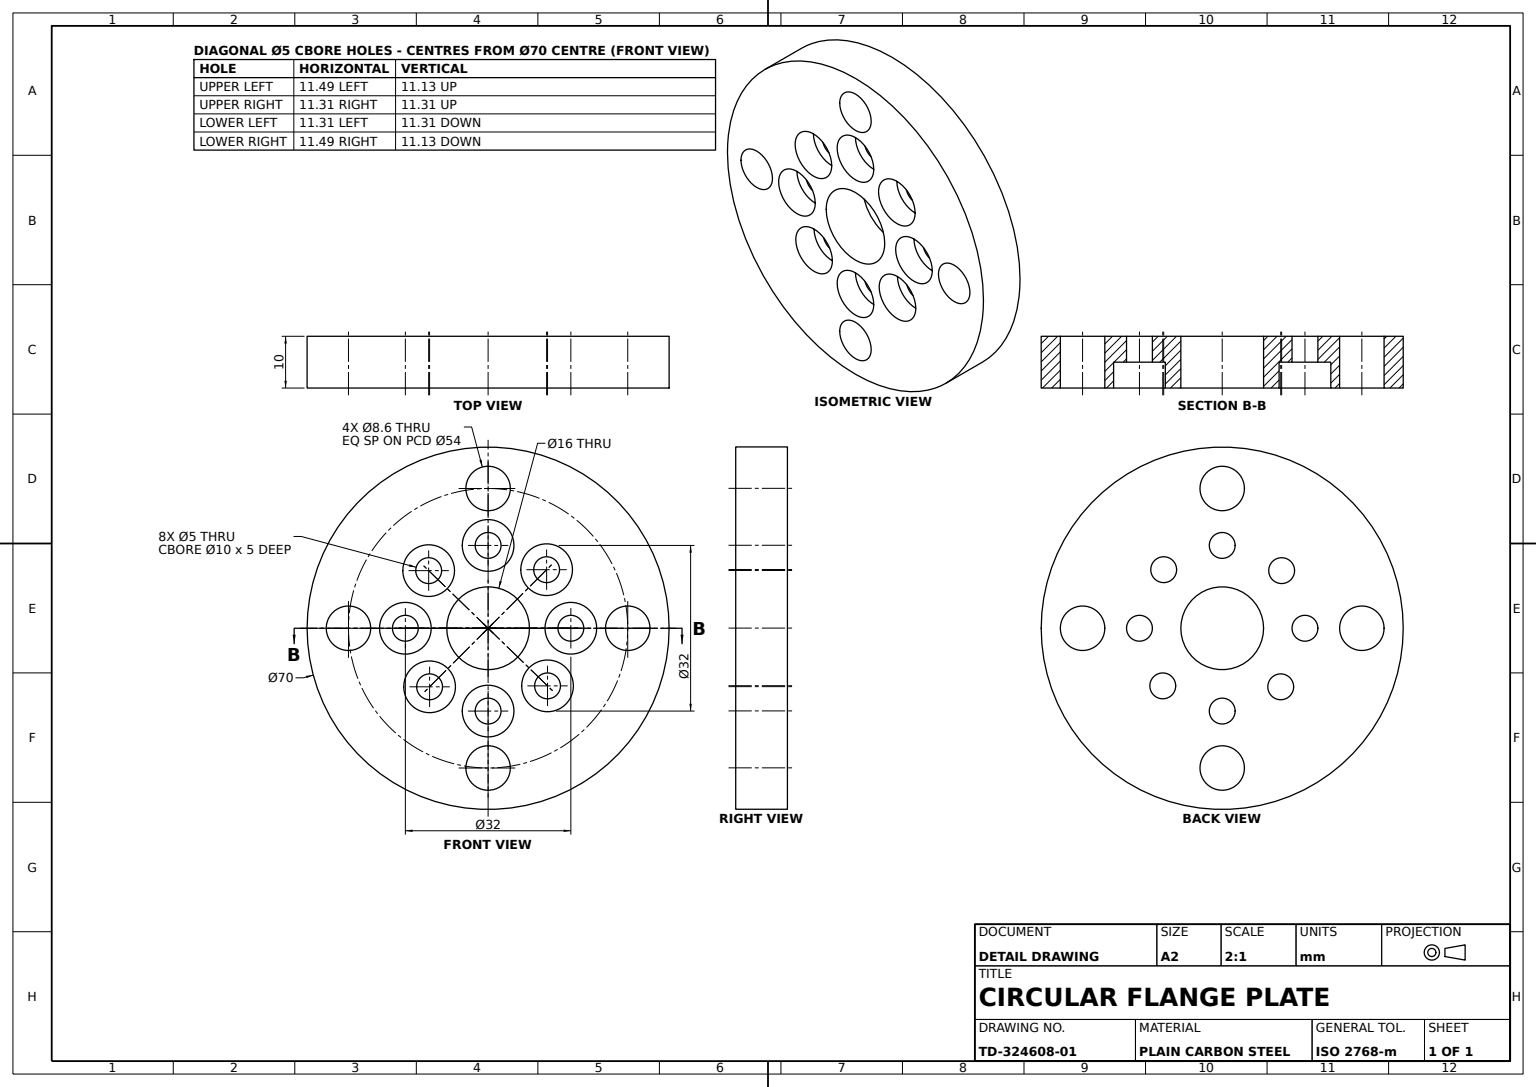
SolidWorks part; units mm, degrees
material "Plain Carbon Steel"
ref_plane "Front Plane" through (0, 0, 0) normal (0, 0, 1) x (1, 0, 0)
ref_plane "Top Plane" through (0, 0, 0) normal (0, 1, 0) x (1, 0, 0)
ref_plane "Right Plane" through (0, 0, 0) normal (1, 0, 0) x (0, 0, -1)
sketch "Disc Profile Ø70" plane through (0, 0, 0) normal (0, 0, 1) x (1, 0, 0)
  circle A0 centre (0, 0) radius 35
  dimension "D1" = 70
  dimension "D2" = 70
extrude "Disc Ø70 x 10" add sketch "Disc Profile Ø70" along normal blind 10
sketch "Centre Bore Profile Ø16" plane through (0, 0, 10) normal (0, 0, 1) x (1, 0, 0)
  circle A0 centre (0, 0) radius 8
  dimension "D1" = 16
  dimension "D2" = 16
extrude "Centre Bore Ø16" cut sketch "Centre Bore Profile Ø16" against normal blind 10
sketch "Outer Holes Profile 4xØ8.6" plane through (0, 0, 10) normal (0, 0, 1) x (1, 0, 0)
  circle A1 centre (0, 27) radius 4.3
  circle A2 centre (27, 0) radius 4.3
  circle A3 centre (0, -27) radius 4.3
  circle A4 centre (-27, 0) radius 4.3
  dimension "D1" = 8.6
  dimension "D2" = 8.6
  dimension "D3" = 8.6
  dimension "D4" = 8.6
  dimension "D5" = 8.6
  dimension "D6" = 27
  dimension "D7" = 27
  dimension "D8" = 27
  dimension "D9" = 27
extrude "Outer Holes 4xØ8.6" cut sketch "Outer Holes Profile 4xØ8.6" against normal blind 10
sketch "Counterbore Profile" plane through (0, 0, 10) normal (0, 0, 1) x (1, 0, 0)
  line L1 (0, 0) -> (0.0257, 0) construction
  line L3 (0, 0) -> (0.0086, 0) construction
  circle A1 centre (0, 16) radius 5
  circle A2 centre (16, 0) radius 5
  circle A3 centre (0, -16) radius 5
  circle A4 centre (-16, 0) radius 5
  circle A5 centre (11.4925, -11.132) radius 5
  circle A6 centre (11.3137, 11.3137) radius 5
  circle A7 centre (-11.4925, 11.132) radius 5
  circle A8 centre (-11.3137, -11.3137) radius 5
  circle A9 centre (0, 27) radius 4.3 construction
  dimension "D1" = 10
  dimension "D2" = 10
  dimension "D3" = 10
  dimension "D4" = 10
  dimension "D5" = 10
  dimension "D6" = 10
  dimension "D7" = 10
  dimension "D8" = 10
  dimension "D9" = 10
  dimension "D10" = 11.3137
  dimension "D11" = 11.4925
  dimension "D12" = 16
  dimension "D13" = 11.3137
  dimension "D14" = 11.4925
  dimension "D15" = 16
  dimension "D16" = 11
  dimension "D17" = 15.6863
  dimension "D18" = 15.868
  dimension "D19" = 38.132
  dimension "D20" = 38.3137
  dimension "D21" = 43
extrude "Counterbores Depth 5" cut sketch "Counterbore Profile" against normal blind 5
sketch "Counterbore Through Hole Profile" plane through (0, 0, 5) normal (0, 0, 1) x (1, 0, 0)
  circle A0 centre (0, 16) radius 2.5
  circle A1 centre (11.3137, 11.3137) radius 2.5
  circle A2 centre (16, 0) radius 2.5
  circle A3 centre (11.4925, -11.132) radius 2.5
  circle A4 centre (0, -16) radius 2.5
  circle A5 centre (-11.3137, -11.3137) radius 2.5
  circle A6 centre (-16, 0) radius 2.5
  circle A7 centre (-11.4925, 11.132) radius 2.5
  dimension "D1" = 5
  dimension "D2" = 5
  dimension "D3" = 5
  dimension "D4" = 2.5
  dimension "D5" = 2.5
  dimension "D6" = 2.5
  dimension "D7" = 2.5
  dimension "D8" = 2.5
  dimension "D9" = 5
extrude "Counterbore Through Holes" cut sketch "Counterbore Through Hole Profile" against normal blind 5
